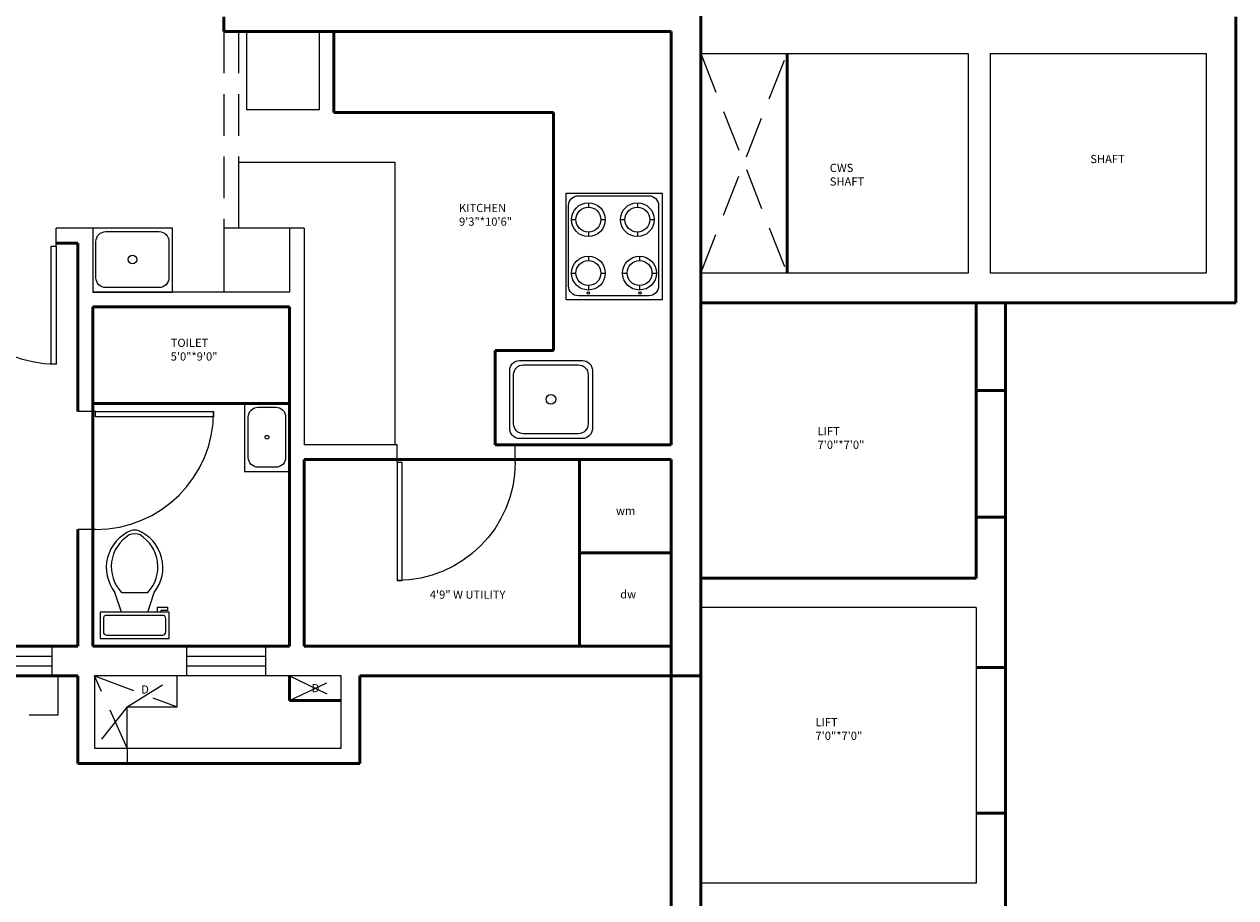
# Model space of a CAD drawing. Units: inches. Extents: x 4795 to 6024, y 2716 to 5025.
# Tile 5 of 19: x 5081 to 5450, y 3283 to 3549. Entities that reach past the tile are written whole.
import ezdxf

# ---------------------------------------------------------------- set-up
doc = ezdxf.new("R2010")
doc.units = ezdxf.units.IN
doc.linetypes.add('DASHED', pattern=[19.05, 12.7, -6.35])
for name, color, linetype, lineweight in [('A-ANNO-TEXT', 7, 'Continuous', 18), ('A-AREA-IDEN', 3, 'Continuous', 18), ('A-DOOR', 4, 'Continuous', 25), ('A-FLOR-FIXT', 9, 'Continuous', 18), ('A-FURN', 8, 'Continuous', 18), ('A-GLAZ', 4, 'Continuous', 25), ('A-WALL', 7, 'Continuous', 50), ('A-WALL-OVHD', 8, 'DASHED', 18)]:
    doc.layers.add(name, color=color, linetype=linetype, lineweight=lineweight)
doc.styles.get("Standard").update_dxf_attribs({"font": 'arial.ttf'})

# ---------------------------------------------------------------- blocks, each defined once
blk = doc.blocks.new('*U2')
for p, q in [((0, 0), (0, -6)), ((40, 0), (40, -6))]:
    blk.add_line(p, q)
blk.add_lwpolyline([(0, 0), (0, 40), (1.75, 40), (1.75, 0)], close=True)
blk.add_arc((0, 0), 40, 0, 90)
blk = doc.blocks.new('Toilet - top')
for p, q in [((9.5, -6), (9.5, -2)), ((-10, -8.5), (-8, -8.5)), ((-10, -9.5), (-10, -8.5)), ((-7, -9.5), (-10, -9.5)), ((-8, -8.5), (-8, -8)), ((-7, -8), (-7, -9.5)), ((-4, -8), (-6, -14)), ((4, -8), (6, -14)), ((4, -14), (-4, -14))]:
    blk.add_line(p, q)
blk.add_lwpolyline([(10.5, -8), (10.5, 0), (-10.5, 0), (-10.5, -8)], close=True)
for points in [[(-9.5, -2), (-9.5, -6)], [(8.5, -1), (-8.5, -1)], [(-8.5, -7), (8.5, -7)]]:
    blk.add_lwpolyline(points)
for centre, radius, start, end in [((-8.62, -1.88), 0.884, 81.8699, 188.1301), ((8.62, -1.88), 0.884, 351.8699, 98.1301), ((-8.62, -6.12), 0.884, 171.8699, 278.1301), ((8.62, -6.12), 0.884, 261.8699, 8.1301), ((3.52, -21.58), 12.17, 141.4691, 247.9714), ((4.2, -21.82), 11.33, 136.3677, 238.9468), ((-3.52, -21.58), 12.17, 292.0284, 38.5307), ((-4.2, -21.82), 11.33, 301.053, 43.6321), ((0, -27.88), 4, 245.7318, 294.2682), ((0, -29), 4, 254.8605, 285.1395)]:
    blk.add_arc(centre, radius, start, end)
blk = doc.blocks.new('WIN-24')
for p, q in [((0, 0), (0, 9)), ((0, 9), (24, 9)), ((24, 9), (24, 0)), ((0, 6), (24, 6)), ((24, 3), (0, 3)), ((24, 0), (0, 0))]:
    blk.add_line(p, q)
blk = doc.blocks.new('COOKTOP-4B')
for p, q in [((6.77, 29.57), (6.77, 28.22)), ((21.7, 29.57), (21.7, 28.22)), ((1.61, 24.41), (2.97, 24.41)), ((10.57, 24.41), (11.93, 24.41)), ((16.54, 24.41), (17.9, 24.41)), ((25.51, 24.41), (26.87, 24.41)), ((6.77, 20.61), (6.77, 19.25)), ((21.7, 20.61), (21.7, 19.25)), ((6.77, 13.27), (6.77, 11.91)), ((22.37, 13.27), (22.37, 11.91)), ((1.61, 8.11), (2.97, 8.11)), ((10.57, 8.11), (11.93, 8.11)), ((17.2, 8.11), (18.56, 8.11)), ((26.17, 8.11), (27.53, 8.11)), ((6.77, 4.3), (6.77, 2.94)), ((22.37, 4.3), (22.37, 2.94))]:
    blk.add_line(p, q)
blk.add_lwpolyline([(0, 32.52), (29.24, 32.52), (29.24, 0), (0, 0)], close=True)
blk.add_lwpolyline([(3.72, 31.71), (25.19, 31.71, -0.414214), (28.19, 28.71), (28.19, 4.17, -0.414214), (25.19, 1.17), (3.72, 1.17, -0.414214), (0.72, 4.17), (0.72, 28.71, -0.414214)], format="xyb", close=True)
for centre, radius in [((6.77, 24.41), 5.16), ((21.7, 24.41), 5.16), ((6.77, 24.41), 3.8), ((21.7, 24.41), 3.8), ((6.77, 8.11), 5.16), ((6.77, 8.11), 3.8), ((22.37, 8.11), 5.16), ((22.37, 8.11), 3.8), ((6.77, 2), 0.353), ((22.47, 2), 0.353)]:
    blk.add_circle(centre, radius)

msp = doc.modelspace()

# ---------------------------------------------------------------- linework, layer by layer
at = {"layer": 'A-FLOR-FIXT'}
for points in [[(5101.47, 3467.43), (5125.85, 3467.43), (5125.85, 3486.92), (5101.47, 3486.92)], [(5161.47, 3433.52), (5147.81, 3433.52), (5147.81, 3412.71), (5161.47, 3412.71)]]:
    msp.add_lwpolyline(points, close=True, dxfattribs=at)
for points in [[(5105.46, 3485.92), (5121.72, 3485.92, -0.414214), (5124.72, 3482.92), (5124.72, 3471.84, -0.414214), (5121.72, 3468.84), (5105.46, 3468.84, -0.414214), (5102.46, 3471.84), (5102.46, 3482.92, -0.414214)], [(5231.7, 3446.6), (5250.91, 3446.6, -0.414214), (5253.91, 3443.6), (5253.91, 3425.81, -0.414214), (5250.91, 3422.81), (5231.7, 3422.81, -0.414214), (5228.7, 3425.81), (5228.7, 3443.6, -0.414214)], [(5232.89, 3445.29), (5249.63, 3445.29, -0.414214), (5252.63, 3442.29), (5252.63, 3427.28, -0.414214), (5249.63, 3424.28), (5232.89, 3424.28, -0.414214), (5229.89, 3427.28), (5229.89, 3442.29, -0.414214)], [(5151.94, 3432.36), (5157.34, 3432.36, -0.414214), (5160.34, 3429.36), (5160.34, 3417.05, -0.414214), (5157.34, 3414.05), (5151.94, 3414.05, -0.414214), (5148.94, 3417.05), (5148.94, 3429.36, -0.414214)]]:
    msp.add_lwpolyline(points, format="xyb", close=True, dxfattribs=at)
for centre, radius in [((5113.59, 3477.38), 1.31), ((5241.26, 3434.79), 1.48), ((5154.64, 3423.2), 0.579)]:
    msp.add_circle(centre, radius, dxfattribs=at)
at = {"layer": 'A-FURN'}
for p, q in [((5286.97, 3540.28), (5368.6, 3540.28)), ((5368.6, 3540.28), (5368.6, 3473.24)), ((5375.31, 3540.28), (5375.31, 3473.24)), ((5375.31, 3540.28), (5441.22, 3540.28)), ((5441.22, 3540.28), (5441.22, 3473.24)), ((5145.97, 3507.07), (5145.97, 3486.93)), ((5145.97, 3507.07), (5193.68, 3507.07)), ((5193.68, 3507.07), (5193.68, 3420.93)), ((5101.47, 3486.93), (5090.35, 3486.93)), ((5101.47, 3486.93), (5101.47, 3467.43)), ((5165.97, 3486.93), (5141.47, 3486.93)), ((5141.47, 3486.93), (5141.47, 3467.43)), ((5161.47, 3486.93), (5161.47, 3467.43)), ((5165.97, 3486.93), (5165.97, 3420.93)), ((5368.6, 3473.24), (5286.97, 3473.24)), ((5441.22, 3473.24), (5375.31, 3473.24)), ((5161.47, 3467.43), (5101.47, 3467.43)), ((5194.36, 3420.93), (5165.97, 3420.93)), ((5370.97, 3371.24), (5286.97, 3371.24)), ((5370.97, 3371.24), (5370.97, 3350.43)), ((5101.97, 3350.43), (5101.97, 3328.36)), ((5177.3, 3350.43), (5101.97, 3350.43)), ((5127.22, 3341.01), (5127.22, 3350.43)), ((5177.3, 3328.36), (5177.3, 3350.43)), ((5370.97, 3350.43), (5370.97, 3287.24)), ((5112.02, 3328.36), (5112.02, 3341.01)), ((5112.02, 3341.01), (5127.22, 3341.01)), ((5101.97, 3328.36), (5177.3, 3328.36)), ((5112.02, 3328.36), (5112.02, 3323.66)), ((5370.97, 3287.24), (5286.97, 3287.24))]:
    msp.add_line(p, q, dxfattribs=at)
msp.add_lwpolyline([(5170.71, 3546.93), (5148.43, 3546.93), (5148.43, 3523.16), (5170.71, 3523.16)], close=True, dxfattribs=at)
at = {"layer": 'A-WALL'}
for p, q in [((5286.97, 3740.43), (5286.97, 3350.43)), ((5141.47, 3551.43), (5141.47, 3546.93)), ((5450.22, 3551.43), (5450.22, 3464.24)), ((5277.97, 3546.93), (5141.47, 3546.93)), ((5175.09, 3522.25), (5175.09, 3546.93)), ((5277.97, 3546.93), (5277.97, 3420.93)), ((5313.35, 3540.28), (5313.35, 3473.24)), ((5242.06, 3522.25), (5175.09, 3522.25)), ((5242.06, 3522.25), (5242.06, 3449.62)), ((5096.97, 3482.43), (5090.35, 3482.43)), ((5096.97, 3482.43), (5096.97, 3431.03)), ((5450.22, 3464.24), (5286.97, 3464.24)), ((5370.97, 3464.24), (5370.97, 3380.24)), ((5379.97, 3464.24), (5379.97, 3350.43)), ((5161.47, 3462.93), (5101.47, 3462.93)), ((5101.47, 3462.93), (5101.47, 3359.43)), ((5161.47, 3462.93), (5161.47, 3359.43)), ((5224.22, 3420.93), (5224.22, 3449.62)), ((5224.22, 3449.62), (5242.06, 3449.62)), ((5370.97, 3437.42), (5379.97, 3437.42)), ((5101.47, 3433.52), (5161.47, 3433.52)), ((5277.97, 3420.93), (5224.22, 3420.93)), ((5277.97, 3416.43), (5165.97, 3416.43)), ((5165.97, 3416.43), (5165.97, 3359.43)), ((5249.99, 3416.43), (5249.99, 3359.43)), ((5277.97, 3416.43), (5277.97, 3359.43)), ((5370.97, 3398.79), (5379.97, 3398.79)), ((5096.97, 3395.03), (5096.97, 3359.43)), ((5249.99, 3387.93), (5277.97, 3387.93)), ((5370.97, 3380.24), (5286.97, 3380.24)), ((5096.97, 3359.43), (4925.97, 3359.43)), ((5161.47, 3359.43), (5101.47, 3359.43)), ((5277.97, 3359.43), (5165.97, 3359.43)), ((5277.97, 3359.43), (5277.97, 2746.24)), ((5370.97, 3353.02), (5379.97, 3353.02)), ((5096.97, 3350.43), (4916.97, 3350.43)), ((5096.97, 3350.43), (5096.97, 3323.66)), ((5161.47, 3350.43), (5161.47, 3342.86)), ((5286.97, 3350.43), (5183, 3350.43)), ((5183, 3323.66), (5183, 3350.43)), ((5286.97, 3350.43), (5286.97, 2746.24)), ((5379.97, 3350.43), (5379.97, 3185.24)), ((5161.47, 3342.86), (5177.3, 3342.86)), ((5096.97, 3323.66), (5183, 3323.66)), ((5370.97, 3308.57), (5379.97, 3308.57))]:
    msp.add_line(p, q, dxfattribs=at)
at = {"layer": 'A-WALL-OVHD'}
for p, q in [((5141.47, 3546.93), (5141.47, 3486.93)), ((5145.97, 3546.93), (5145.97, 3507.07)), ((5286.97, 3540.28), (5313.35, 3473.24)), ((5286.97, 3473.24), (5313.35, 3540.28)), ((5090.95, 3338.54), (5090.95, 3350.43)), ((5101.97, 3350.43), (5127.22, 3341.01)), ((5112.02, 3328.36), (5101.97, 3350.43)), ((5112.02, 3341.01), (5127.22, 3350.43)), ((5161.47, 3350.43), (5177.3, 3342.86)), ((5161.47, 3342.86), (5177.3, 3350.43)), ((5062.99, 3338.54), (5090.95, 3338.54)), ((5112.02, 3341.01), (5101.97, 3328.36))]:
    msp.add_line(p, q, dxfattribs=at)

# ---------------------------------------------------------------- block references
at = {"layer": 'A-DOOR', "yscale": 0.9, "zscale": 0.9}
for p, xscale, rotation in [((5090.35, 3481.53), 0.9, 180), ((5102.37, 3431.03), 0.9, 270), ((5194.36, 3415.53), -0.9, 180)]:
    msp.add_blockref('*U2', p, dxfattribs=dict(at, xscale=xscale, rotation=rotation))
at = {"layer": 'A-FLOR-FIXT'}
msp.add_blockref('COOKTOP-4B', (5245.94, 3465.16), dxfattribs=at)
at = {"layer": 'A-FLOR-FIXT', "rotation": 180}
msp.add_blockref('Toilet - top', (5114.26, 3361.86), dxfattribs=at)
at = {"layer": 'A-GLAZ', "rotation": 180}
for p in [(5088.95, 3359.43), (5154.16, 3359.43)]:
    msp.add_blockref('WIN-24', p, dxfattribs=at)

# ---------------------------------------------------------------- texts
at = {"layer": 'A-ANNO-TEXT', "char_height": 2.5, "attachment_point": 1}
for s, width, insert in [('wm', 13.3631, (5261.13, 3402.03)), ('dw', 12.8823, (5262.41, 3376.55)), ('D', 2.0223, (5116.27, 3347.52)), ('D', 2.6182, (5168.27, 3347.91))]:
    msp.add_mtext_dynamic_manual_height_columns(s, width=width, gutter_width=12.5, heights=[0], dxfattribs=dict(at, insert=insert))
at = {"layer": 'A-AREA-IDEN', "char_height": 2.5, "attachment_point": 1}
for s, width, insert in [('SHAFT', 33.5789, (5405.84, 3509.31)), ('CWS\\PSHAFT', 38.9888, (5326.35, 3506.61)), ('KITCHEN\\P9\'3"*10\'6"', 38.5801, (5213.23, 3494.38)), ('TOILET\\P5\'0"*9\'0"', 44.499, (5125.26, 3453.25)), ('LIFT\\P7\'0"*7\'0"', 47.1279, (5322.62, 3426.32)), ('4\'9" W UTILITY', 54.9271, (5204.31, 3376.45)), ('LIFT\\P7\'0"*7\'0"', 36.1858, (5321.99, 3337.57))]:
    msp.add_mtext_dynamic_manual_height_columns(s, width=width, gutter_width=12.5, heights=[0], dxfattribs=dict(at, insert=insert))

doc.saveas('drawing.dxf')
